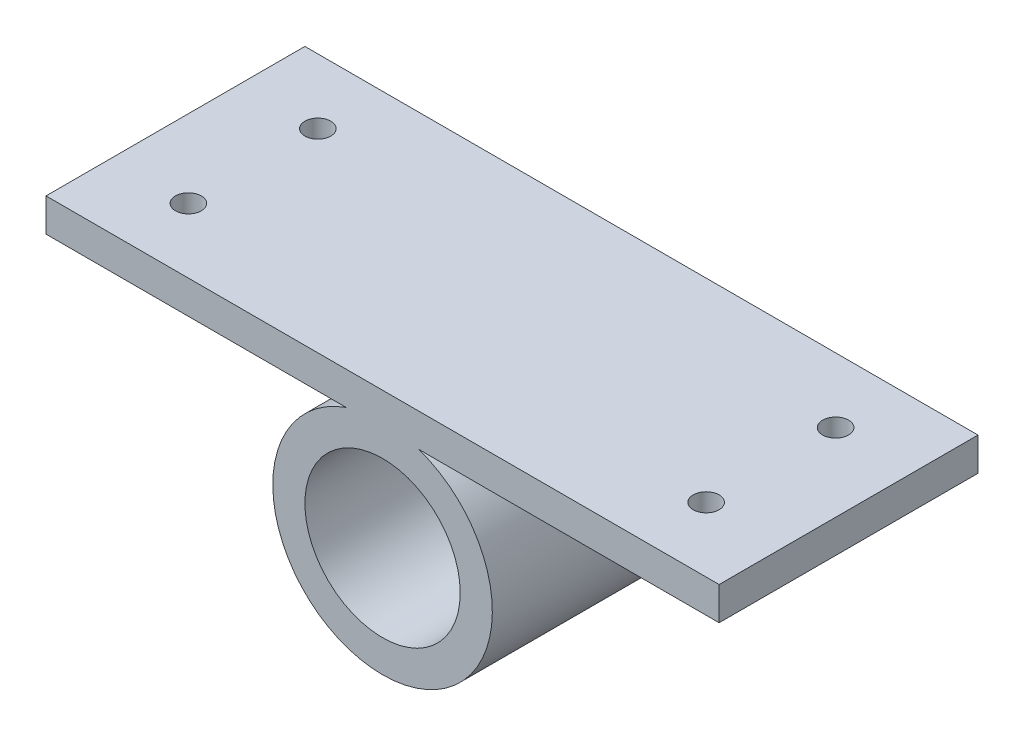
from build123d import *

# Parameters (mm, degrees)
PLATE_AND_TUBE_PROFILE_SKETCH_R = 75
PLATE_AND_TUBE_BODY_DEPTH       = 250
MOUNTING_HOLES_4X_REACH         = 476.098
MOUNTING_HOLES_SKETCH_R         = 12.5


with BuildPart() as part:
    # Plate and Tube Profile Sketch → Plate and Tube Body (new body)
    with BuildSketch(Plane.XY):
        with BuildLine():
            Line((35.156791662, -16), (325, -16))
            Line((325, -16), (325, 16))
            Line((325, 16), (-325, 16))
            Line((-325, 16), (-325, -16))
            Line((-325, -16), (-35.156791662, -16))
            ThreePointArc((-35.156791662, -16), (0, -222), (35.156791662, -16))
        make_face()
        with Locations((0, -116)):
            Circle(PLATE_AND_TUBE_PROFILE_SKETCH_R, mode=Mode.SUBTRACT)
    extrude(amount=PLATE_AND_TUBE_BODY_DEPTH)

    # Mounting Holes Sketch → Mounting Holes 4x (cut, up to next)
    with BuildSketch(Plane(origin=(0, 16, 0), x_dir=(1, 0, 0), z_dir=(0, 1, 0)), mode=Mode.PRIVATE) as mounting_holes_4x_sk1:
        with Locations(Location((-250, -62.5, 0), (0, 0, 270))):
            Circle(MOUNTING_HOLES_SKETCH_R)
    mounting_holes_4x_tool1 = extrude(mounting_holes_4x_sk1.sketch, amount=-MOUNTING_HOLES_4X_REACH, mode=Mode.PRIVATE) & part.part
    # Mounting Holes Sketch → Mounting Holes 4x (cut, up to next)
    with BuildSketch(Plane(origin=(0, 16, 0), x_dir=(1, 0, 0), z_dir=(0, 1, 0)), mode=Mode.PRIVATE) as mounting_holes_4x_sk2:
        with Locations(Location((250, -62.5, 0), (0, 0, 270))):
            Circle(MOUNTING_HOLES_SKETCH_R)
    mounting_holes_4x_tool2 = extrude(mounting_holes_4x_sk2.sketch, amount=-MOUNTING_HOLES_4X_REACH, mode=Mode.PRIVATE) & part.part
    # Mounting Holes Sketch → Mounting Holes 4x (cut, up to next)
    with BuildSketch(Plane(origin=(0, 16, 0), x_dir=(1, 0, 0), z_dir=(0, 1, 0)), mode=Mode.PRIVATE) as mounting_holes_4x_sk3:
        with Locations(Location((-250, -187.5, 0), (0, 0, 270))):
            Circle(MOUNTING_HOLES_SKETCH_R)
    mounting_holes_4x_tool3 = extrude(mounting_holes_4x_sk3.sketch, amount=-MOUNTING_HOLES_4X_REACH, mode=Mode.PRIVATE) & part.part
    # Mounting Holes Sketch → Mounting Holes 4x (cut, up to next)
    with BuildSketch(Plane(origin=(0, 16, 0), x_dir=(1, 0, 0), z_dir=(0, 1, 0)), mode=Mode.PRIVATE) as mounting_holes_4x_sk4:
        with Locations(Location((250, -187.5, 0), (0, 0, 270))):
            Circle(MOUNTING_HOLES_SKETCH_R)
    mounting_holes_4x_tool4 = extrude(mounting_holes_4x_sk4.sketch, amount=-MOUNTING_HOLES_4X_REACH, mode=Mode.PRIVATE) & part.part
    add(mounting_holes_4x_tool1.solids().sort_by_distance((-250, 16, 62.5))[0], mode=Mode.SUBTRACT)
    add(mounting_holes_4x_tool2.solids().sort_by_distance((250, 16, 62.5))[0], mode=Mode.SUBTRACT)
    add(mounting_holes_4x_tool3.solids().sort_by_distance((-250, 16, 187.5))[0], mode=Mode.SUBTRACT)
    add(mounting_holes_4x_tool4.solids().sort_by_distance((250, 16, 187.5))[0], mode=Mode.SUBTRACT)


solid = part.part
